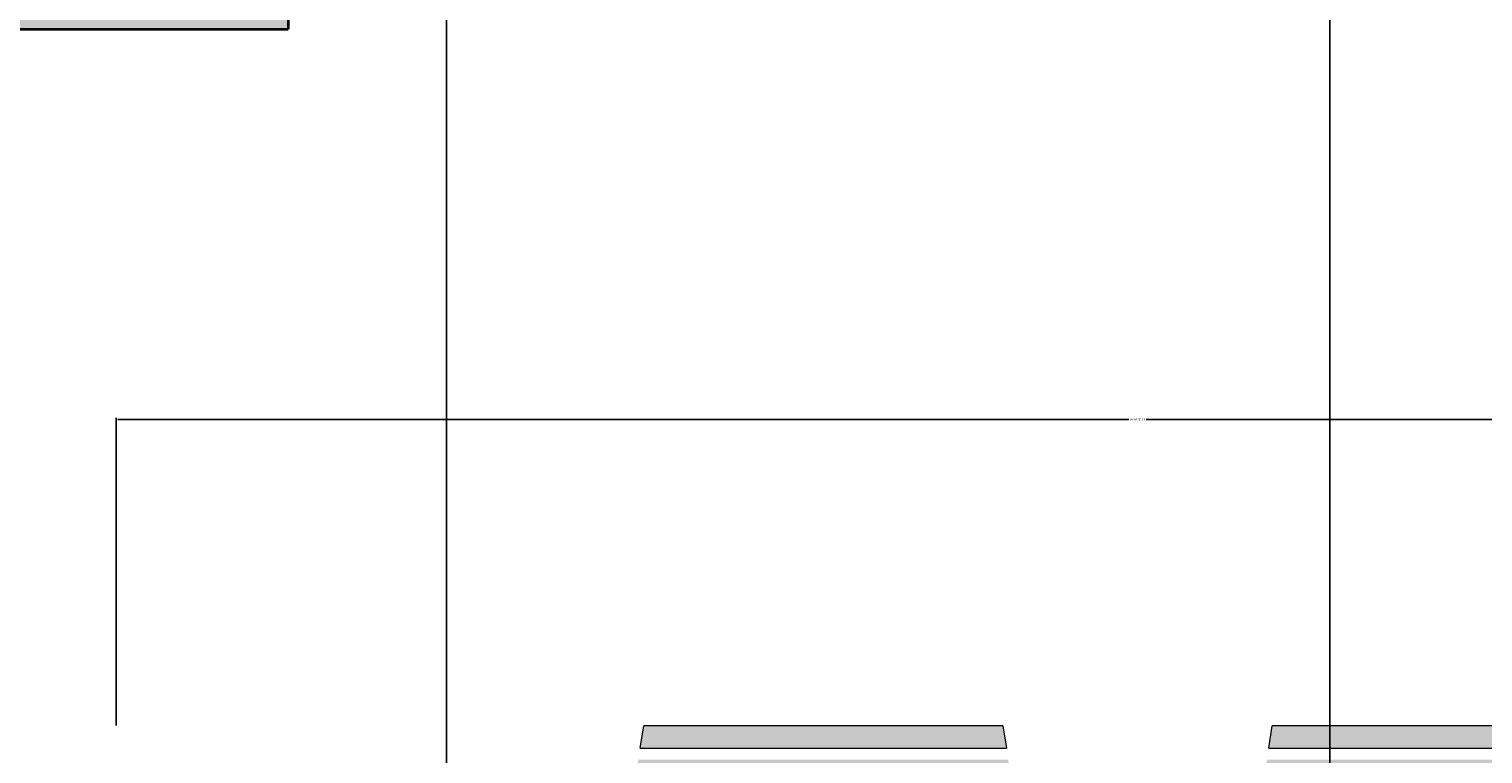
# Model space of a CAD drawing. Units: inches. Extents: x 192 to 1361, y -1362 to 367.
# Tile 17 of 23: x 487 to 662, y -214 to -127. Entities that reach past the tile are written whole.
import ezdxf

# ---------------------------------------------------------------- set-up
doc = ezdxf.new("R2010")
doc.units = ezdxf.units.IN
doc.header["$MEASUREMENT"] = 0
for name, color, linetype, lineweight in [('A-ANNO-DIMS', 2, 'Continuous', 18), ('A-WALL-PATT', 250, 'Continuous', 13), ('furniture', 32, 'Continuous', 18), ('walls', 7, 'Continuous', 35)]:
    doc.layers.add(name, color=color, linetype=linetype, lineweight=lineweight)
doc.layers.add('A-FURN-PATT', color=254, linetype='Continuous', lineweight=13, true_color=0xfeeab9)
doc.styles.get("Standard").update_dxf_attribs({"font": 'arial.ttf'})
doc.dimstyles.get("Standard").update_dxf_attribs({"dimtxt": 0.18, "dimasz": 0.18, "dimexe": 0.18, "dimexo": 0.0625, "dimgap": 0.09, "dimtad": 0, "dimtih": 1, "dimtoh": 1, "dimzin": 0, "dimdsep": 46, "dimlunit": 3, "dimtxsty": 'Standard', "dimcen": 0.09, "dimadec": 0, "dimazin": 0, "dimtfac": 1, "dimtofl": 0, "dimtmove": 0, "dimatfit": 3, "dimfxl": 1, "dimtolj": 1, "dimtzin": 0, "dimarcsym": 0})

# ---------------------------------------------------------------- blocks, each defined once
blk = doc.blocks.new('Dining Set - 36 x 72 in.')
for p, q in [((-5.8416, -26.5), (-22.1534, -26.5)), ((-5.8437, -26.49967), (-6, -27.5)), ((6, -27.5), (5.8438, -26.50044)), ((22.1584, -26.5), (5.8466, -26.5)), ((22.1563, -26.49967), (22, -27.5)), ((-22, -27.5), (-6, -27.5)), ((6, -27.5), (22, -27.5))]:
    blk.add_line(p, q)
blk = doc.blocks.new('dining area')
at = {"layer": 'furniture', "xscale": 0.6659924291999282, "yscale": 0.6659924291999282, "zscale": 0.6659924291999282, "rotation": 90}
blk.add_blockref('Dining Set - 36 x 72 in.', (-0.439, 20.507), dxfattribs=at)
blk = doc.blocks.new('*D43')
at = {"layer": 'A-ANNO-DIMS', "color": 0, "lineweight": -2, "transparency": 16777216}
for p, q in [((497.85, -210.68), (497.85, -173.69)), ((498.03, -173.87), (619.71, -173.87)), ((743.46, -173.87), (621.79, -173.87)), ((743.64, -210.68), (743.64, -173.69))]:
    blk.add_line(p, q, dxfattribs=at)
at = {"layer": 'A-ANNO-DIMS', "color": 0, "transparency": 16777216}
for points in [[(498.03, -173.84), (498.03, -173.9), (497.85, -173.87)], [(743.46, -173.84), (743.46, -173.9), (743.64, -173.87)]]:
    blk.add_solid(points, dxfattribs=at)
at = {"layer": 'Defpoints', "color": 0, "transparency": 16777216}
for p in [(497.85, -173.87), (497.85, -210.74), (743.64, -210.74)]:
    blk.add_point(p, dxfattribs=at)
at = {"layer": 'A-ANNO-DIMS', "color": 0, "transparency": 16777216, "insert": (620.75, -173.87), "char_height": 0.18, "attachment_point": 5}
blk.add_mtext('\\A1;DINING SET 246', dxfattribs=at)
blk = doc.blocks.new('*D70')
at = {"layer": 'A-ANNO-DIMS', "color": 0, "lineweight": -2, "transparency": 16777216}
for p, q in [((537.57, -441.84), (537.57, 367.39)), ((643.89, -441.84), (643.89, 367.39)), ((537.75, 367.21), (590.28, 367.21)), ((643.71, 367.21), (591.19, 367.21))]:
    blk.add_line(p, q, dxfattribs=at)
at = {"layer": 'A-ANNO-DIMS', "color": 0, "transparency": 16777216}
for points in [[(537.75, 367.24), (537.75, 367.18), (537.57, 367.21)], [(643.71, 367.24), (643.71, 367.18), (643.89, 367.21)]]:
    blk.add_solid(points, dxfattribs=at)
at = {"layer": 'Defpoints', "color": 0, "transparency": 16777216}
for p in [(643.89, 367.21), (537.57, -441.9), (643.89, -441.9)]:
    blk.add_point(p, dxfattribs=at)
at = {"layer": 'A-ANNO-DIMS', "color": 0, "transparency": 16777216, "insert": (590.73, 367.21), "char_height": 0.18, "attachment_point": 5}
blk.add_mtext('\\A1;106.32', dxfattribs=at)

msp = doc.modelspace()

# ---------------------------------------------------------------- hatches: boundary and pattern name
at = {"layer": 'A-FURN-PATT'}
h = msp.add_hatch(color=256, dxfattribs=at)
h.dxf.hatch_style = 1
h.paths.add_polyline_path([(605.1742, -214.7906), (560.6934, -214.7906), (557.3171, -236.398), (608.5502, -236.398)])
h.paths.add_polyline_path([(604.5412, -210.7392), (561.3264, -210.7392), (560.9044, -213.4402), (604.9632, -213.4402)])
h.paths.add_polyline_path([(680.8, -214.7906), (636.3191, -214.7906), (632.9429, -236.398), (684.176, -236.398)])
h.paths.add_polyline_path([(680.1669, -210.7392), (636.9522, -210.7392), (636.5302, -213.4402), (680.589, -213.4402)])
h.paths.add_polyline_path([(523.5135, -259.398), (501.9062, -262.7741), (501.9062, -307.2549), (523.5135, -310.6311)])
h.paths.add_polyline_path([(500.5557, -262.9851), (497.8548, -263.4072), (497.8548, -306.6219), (500.5557, -307.0439)])
h.paths.add_polyline_path([(608.5502, -333.6311), (557.3171, -333.6311), (560.6934, -355.2385), (605.1742, -355.2385)])
h.paths.add_polyline_path([(604.9632, -356.5889), (560.9044, -356.5889), (561.3264, -359.2899), (604.5412, -359.2899)])
h.paths.add_polyline_path([(680.589, -356.5889), (636.5302, -356.5889), (636.9522, -359.2899), (680.1669, -359.2899)])
h.paths.add_polyline_path([(684.176, -333.6311), (632.9429, -333.6311), (636.3191, -355.2385), (680.8, -355.2385)])
h.paths.add_polyline_path([(739.5872, -262.7741), (717.9798, -259.398), (717.9798, -310.6311), (739.5872, -307.2549)])
h.paths.add_polyline_path([(743.6386, -263.4072), (740.9376, -262.9851), (740.9376, -307.0439), (743.6386, -306.6219)])
at = {"layer": 'A-WALL-PATT'}
h = msp.add_hatch(color=256, dxfattribs=at)
h.dxf.hatch_style = 1
h.paths.add_polyline_path([(309.5452, 191.102), (300.5452, 191.102), (300.5452, -126.898), (309.5452, -126.898), (309.5452, -117.898)])
h.paths.add_polyline_path([(420.798, 191.102), (337.3229, 191.102), (337.3229, 182.102), (420.798, 182.102)])
h.paths.add_polyline_path([(518.5452, 182.102), (625.4022, 182.102), (625.4022, 191.102), (509.5452, 191.102), (509.5452, 114.3262), (518.5452, 114.3262)])
h.paths.add_polyline_path([(842.5452, 191.102), (763.4438, 191.102), (763.4438, 182.102), (833.5452, 182.102), (833.5452, 161.1615), (836.8088, 161.1615), (842.5452, 161.1615)])
h.paths.add_polyline_path([(842.5452, -16.5675), (833.5452, -16.5675), (833.5452, -60.4996), (784.8041, -60.4996), (784.8041, -354.6796), (793.8041, -354.6796), (793.8041, -69.4996), (1094.1252, -69.4996), (1094.1252, -60.4996), (842.5452, -60.4996)])
h.paths.add_polyline_path([(518.5452, 36.602), (509.5452, 36.602), (509.5452, -117.898), (420.2204, -117.898), (420.2204, -126.898), (518.5452, -126.898)])
h.paths.add_polyline_path([(474.8041, -377.0384), (465.8041, -377.0384), (465.8041, -381.5384), (465.8041, -450.898), (537.5717, -450.898), (537.5717, -441.898), (474.8041, -441.898)])
h.paths.add_polyline_path([(1162.8041, -380.6763), (1204.3001, -380.6763), (1204.3001, -375.6763), (1195.1471, -375.6763), (1153.8041, -375.6763), (1153.8041, -448.4996), (856.5691, -448.4996), (856.5691, -457.4996), (1162.8041, -457.4996)])
h.paths.add_polyline_path([(1162.8041, -525.128), (1153.8041, -525.128), (1153.8041, -597.4996), (1162.8041, -597.4996)], flags=17)
h.paths.add_polyline_path([(1162.8041, -60.4996), (1153.8041, -60.4996), (1153.8041, -69.4996), (1153.8041, -177.4733), (1205.8889, -177.4733), (1205.8889, -172.4733), (1162.8041, -172.4733)])
h.paths.add_polyline_path([(980.5799, -525.686), (971.5799, -525.686), (971.5799, -597.4996), (980.5799, -597.4996)], flags=17)
h.paths.add_polyline_path([(856.5691, -448.4996), (798.7542, -448.4996), (784.8041, -448.4996), (784.8041, -457.4996), (847.5691, -457.4996), (847.5691, -597.4996), (784.8041, -597.4996), (784.8041, -606.4996), (1273.5658, -606.4996), (1273.5658, -597.4996), (856.5691, -597.4996)])
h.paths.add_polyline_path([(1273.5658, -773.892), (1099.8366, -773.892), (1099.8366, -851.9362), (1108.8366, -851.9362), (1108.8366, -782.892), (1273.5658, -782.892)])
h.paths.add_polyline_path([(1108.8366, -982.9214), (1099.8366, -982.9214), (1099.8366, -1067.6246), (1037.7563, -1067.6246), (1037.7563, -1076.6246), (1108.8366, -1076.6246)])
h.paths.add_polyline_path([(835.078, -1067.6246), (758.8458, -1067.6246), (758.8458, -940.2324), (749.8458, -940.2324), (749.8458, -963.172), (749.8458, -970.4644), (749.8458, -1076.6246), (835.078, -1076.6246)])
h.paths.add_polyline_path([(450.307, -1066.9838), (441.307, -1066.9838), (441.307, -1076.6246), (450.307, -1076.6246)])
h.paths.add_polyline_path([(492.8925, -756.4415), (274.8925, -756.4415), (274.8925, -765.4415), (492.8925, -765.4415)])
h.paths.add_polyline_path([(283.8925, -835.2244), (274.8925, -835.2244), (274.8925, -914.4415), (492.8925, -914.4415), (492.8925, -839.9415), (483.8925, -839.9415), (483.8925, -905.4415), (283.8925, -905.4415)])
h.paths.add_polyline_path([(283.8925, -441.898), (283.8925, -375.4296), (281.6021, -375.4296), (281.6021, -399.4121), (274.8925, -399.4121), (274.8925, -441.898), (274.8925, -684.5089), (283.8925, -684.5089)])

# ---------------------------------------------------------------- linework, layer by layer
at = {"layer": 'walls'}
for p in [(518.5452, 36.602), (300.5452, -126.898)]:
    msp.add_line(p, (518.5452, -126.898), dxfattribs=at)

# ---------------------------------------------------------------- block references
at = {"layer": 'furniture', "xscale": 4.055482377011951, "yscale": 4.055482377011951, "zscale": 4.055482377011951, "rotation": 90}
msp.add_blockref('dining area', (703.9121, -283.2344), dxfattribs=at)

# ---------------------------------------------------------------- dimensions: what is measured, and where the dimension line sits
at = {"layer": 'A-ANNO-DIMS'}
dim = msp.add_linear_dim(base=(643.8925, 367.2097), p1=(537.5717, -441.898), p2=(643.8925, -441.898), dimstyle='Standard', override={"dimdec": 2, "dimlfac": 1, "dimrnd": 0, "dimzin": 0, "dimdsep": 46, "dimlunit": 2}, dxfattribs=at)
dim.commit()
dim.dimension.update_dxf_attribs({"geometry": '*D70', "text_midpoint": (590.7321, 367.2097)})
dim = msp.add_linear_dim(base=(497.8548, -173.8717), p1=(743.6386, -210.7392), p2=(497.8548, -210.7392), angle=180, text='DINING SET <>', dimstyle='Standard', override={"dimdec": 0, "dimlfac": 1, "dimrnd": 0, "dimzin": 0, "dimdsep": 46, "dimlunit": 2}, dxfattribs=at)
dim.commit()
dim.dimension.update_dxf_attribs({"geometry": '*D43', "text_midpoint": (620.7467, -173.8717)})

doc.saveas('drawing.dxf')
